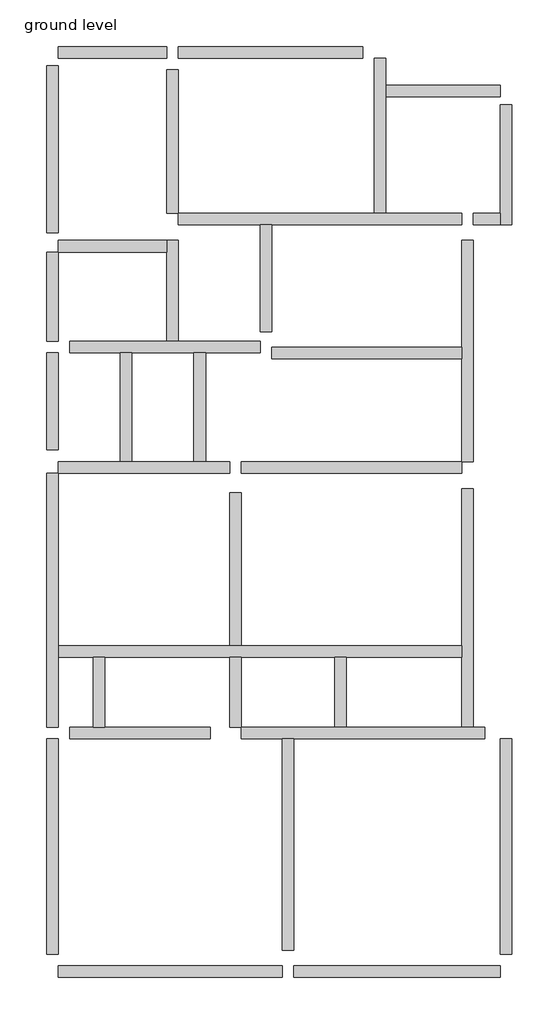
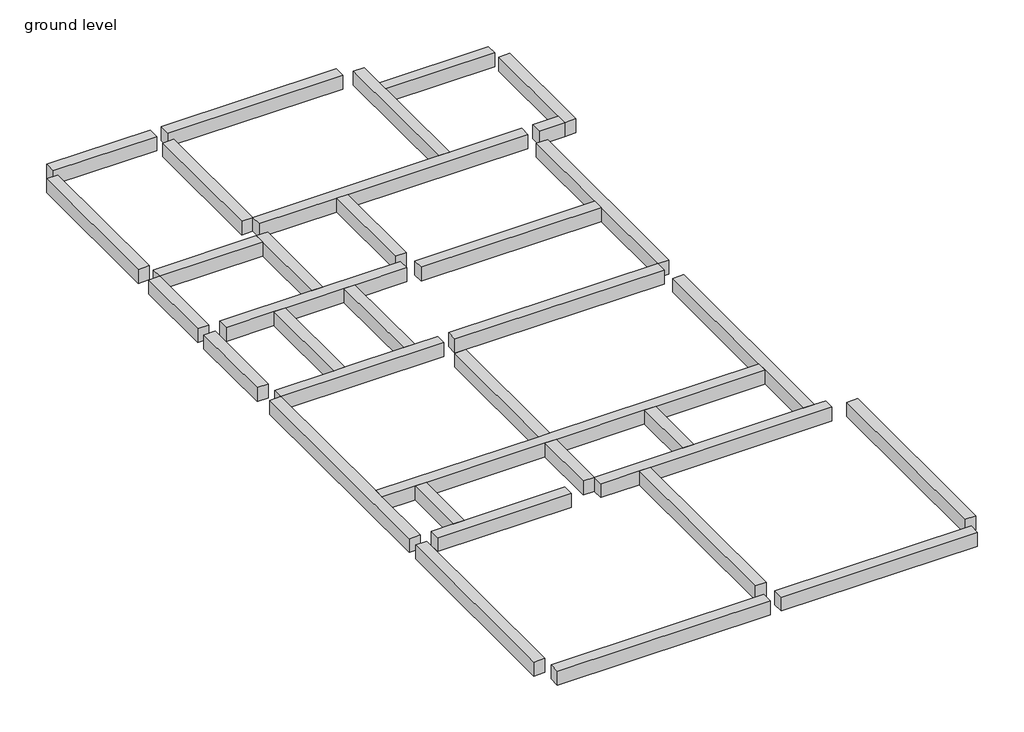
# One storey: 35 beams.
"""IFC4 building model written with IfcOpenShell, lengths in millimetres."""

from ifc_helpers import new_model, si_unit, frame, origin, place, context, project, spatial, polyline, outline, extrude, faceted_brep, element, save

model = new_model("IFC4")

# Units and contexts
model_context = context("Model", 3, world=origin())
ifc_project = project(units=[si_unit("LENGTHUNIT", "METRE", prefix="MILLI")], contexts=[model_context])

# Site, building, storey
site = spatial("IfcSite", under=ifc_project)
building = spatial("IfcBuilding", under=site)
storey = spatial("IfcBuildingStorey", under=building, Name="ground level", Elevation=0.0)

# Beams
placement = place(None, origin())
element("IfcBeam", 1, ObjectType="M_Concrete-Rectangular Beam : 9\" x 12\"", at=placement, inside=storey, context=model_context, shape_type="SweptSolid", body=[
    extrude(outline(polyline([(17883.586814, 18917.5317951), (17654.986814, 18917.5317951), (17654.986814, 22194.1317951), (17883.586814, 22194.1317951), (17883.586814, 18917.5317951)])), frame((0.0, 0.0, -304.8), z_axis=(0.0, 0.0, 1.0), x_axis=(1.0, 0.0, 0.0)), (0.0, 0.0, 1.0), 304.8),
])
element("IfcBeam", 2, ObjectType="M_Concrete-Rectangular Beam : 9\" x 12\"", at=placement, inside=storey, context=model_context, shape_type="SweptSolid", body=[
    extrude(outline(polyline([(20017.186814, 22575.1317951), (20017.186814, 22346.5317951), (17883.586814, 22346.5317951), (17883.586814, 22575.1317951), (20017.186814, 22575.1317951)])), frame((0.0, 0.0, -304.8), z_axis=(0.0, 0.0, 1.0), x_axis=(1.0, 0.0, 0.0)), (0.0, 0.0, 1.0), 304.8),
])
element("IfcBeam", 3, ObjectType="M_Concrete-Rectangular Beam : 9\" x 12\"", at=placement, inside=storey, context=model_context, shape_type="SweptSolid", body=[
    extrude(outline(polyline([(23864.8020345, 22575.1317951), (23864.8020345, 22346.5317951), (20245.786814, 22346.5317951), (20245.786814, 22575.1317951), (23864.8020345, 22575.1317951)])), frame((0.0, 0.0, -304.8), z_axis=(0.0, 0.0, 1.0), x_axis=(1.0, 0.0, 0.0)), (0.0, 0.0, 1.0), 304.8),
])
element("IfcBeam", 4, ObjectType="M_Concrete-Rectangular Beam : 9\" x 12\"", at=placement, inside=storey, context=model_context, shape_type="Brep", body=[
    faceted_brep([(26798.986814, 21432.1317951, 0.0), (26798.986814, 21432.1317951, -304.8), (26570.386814, 21432.1317951, -304.8), (26570.386814, 21432.1317951, 0.0), (26570.386814, 19298.5317951, 0.0), (26570.386814, 19069.9317951, 0.0), (26798.986814, 19069.9317951, 0.0), (26570.386814, 19298.5317951, -304.8), (26570.386814, 19069.9317951, -304.8), (26798.986814, 19069.9317951, -304.8)], [[[0, 1, 2, 3]], [[0, 3, 4, 5, 6]], [[3, 2, 7, 8, 5, 4]], [[2, 1, 9, 8, 7]], [[1, 0, 6, 9]], [[6, 5, 8, 9]]]),
])
element("IfcBeam", 5, ObjectType="M_Concrete-Rectangular Beam : 9\" x 12\"", at=placement, inside=storey, context=model_context, shape_type="SweptSolid", body=[
    extrude(outline(polyline([(26036.986814, 19069.9317951), (26036.986814, 19298.5317951), (26570.386814, 19298.5317951), (26570.386814, 19069.9317951), (26036.986814, 19069.9317951)])), frame((0.0, 0.0, -304.8), z_axis=(0.0, 0.0, 1.0), x_axis=(1.0, 0.0, 0.0)), (0.0, 0.0, 1.0), 304.8),
])
element("IfcBeam", 6, ObjectType="M_Concrete-Rectangular Beam : 9\" x 12\"", at=placement, inside=storey, context=model_context, shape_type="Brep", body=[
    faceted_brep([(20245.786814, 19298.5317951, 0.0), (20245.786814, 19069.9317951, 0.0), (21851.7441916, 19069.9317951, 0.0), (22080.3441916, 19069.9317951, 0.0), (25808.386814, 19069.9317951, 0.0), (25808.386814, 19298.5317951, 0.0), (24318.986814, 19298.5317951, 0.0), (24090.386814, 19298.5317951, 0.0), (20245.786814, 19298.5317951, -304.8), (25808.386814, 19298.5317951, -304.8), (24318.986814, 19298.5317951, -304.8), (24090.386814, 19298.5317951, -304.8), (20245.786814, 19069.9317951, -304.8), (25808.386814, 19069.9317951, -304.8), (22080.3441916, 19069.9317951, -304.8), (21851.7441916, 19069.9317951, -304.8)], [[[0, 1, 2, 3, 4, 5, 6, 7]], [[8, 0, 7, 6, 5, 9, 10, 11]], [[12, 8, 11, 10, 9, 13, 14, 15]], [[1, 12, 15, 14, 13, 4, 3, 2]], [[1, 0, 8, 12]], [[4, 13, 9, 5]]]),
])
element("IfcBeam", 7, ObjectType="M_Concrete-Rectangular Beam : 9\" x 12\"", at=placement, inside=storey, context=model_context, shape_type="SweptSolid", body=[
    extrude(outline(polyline([(20245.786814, 19298.5317951), (20017.186814, 19298.5317951), (20017.186814, 22117.9317951), (20245.786814, 22117.9317951), (20245.786814, 19298.5317951)])), frame((0.0, 0.0, -304.8), z_axis=(0.0, 0.0, 1.0), x_axis=(1.0, 0.0, 0.0)), (0.0, 0.0, 1.0), 304.8),
])
element("IfcBeam", 8, ObjectType="M_Concrete-Rectangular Beam : 9\" x 12\"", at=placement, inside=storey, context=model_context, shape_type="SweptSolid", body=[
    extrude(outline(polyline([(17883.586814, 16783.9317951), (17654.986814, 16783.9317951), (17654.986814, 18536.5317951), (17883.586814, 18536.5317951), (17883.586814, 16783.9317951)])), frame((0.0, 0.0, -304.8), z_axis=(0.0, 0.0, 1.0), x_axis=(1.0, 0.0, 0.0)), (0.0, 0.0, 1.0), 304.8),
])
element("IfcBeam", 9, ObjectType="M_Concrete-Rectangular Beam : 9\" x 12\"", at=placement, inside=storey, context=model_context, shape_type="SweptSolid", body=[
    extrude(outline(polyline([(17883.586814, 14650.3317951), (17654.986814, 14650.3317951), (17654.986814, 16555.3317951), (17883.586814, 16555.3317951), (17883.586814, 14650.3317951)])), frame((0.0, 0.0, -304.8), z_axis=(0.0, 0.0, 1.0), x_axis=(1.0, 0.0, 0.0)), (0.0, 0.0, 1.0), 304.8),
])
element("IfcBeam", 10, ObjectType="M_Concrete-Rectangular Beam : 9\" x 12\"", at=placement, inside=storey, context=model_context, shape_type="Brep", body=[
    faceted_brep([(17654.986814, 9202.0317951, 0.0), (17883.586814, 9202.0317951, 0.0), (17883.586814, 10573.4317951, 0.0), (17883.586814, 10802.0317951, 0.0), (17883.586814, 14193.1317951, 0.0), (17654.986814, 14193.1317951, 0.0), (17654.986814, 9202.0317951, -304.8), (17654.986814, 14193.1317951, -304.8), (17883.586814, 9202.0317951, -304.8), (17883.586814, 14193.1317951, -304.8), (17883.586814, 10802.0317951, -304.8), (17883.586814, 10573.4317951, -304.8)], [[[0, 1, 2, 3, 4, 5]], [[6, 0, 5, 7]], [[8, 6, 7, 9, 10, 11]], [[1, 8, 11, 10, 9, 4, 3, 2]], [[1, 0, 6, 8]], [[4, 9, 7, 5]]]),
])
element("IfcBeam", 11, ObjectType="M_Concrete-Rectangular Beam : 9\" x 12\"", at=placement, inside=storey, context=model_context, shape_type="SweptSolid", body=[
    extrude(outline(polyline([(17883.586814, 4744.3317951), (17654.986814, 4744.3317951), (17654.986814, 8973.4317951), (17883.586814, 8973.4317951), (17883.586814, 4744.3317951)])), frame((0.0, 0.0, -304.8), z_axis=(0.0, 0.0, 1.0), x_axis=(1.0, 0.0, 0.0)), (0.0, 0.0, 1.0), 304.8),
])
element("IfcBeam", 12, ObjectType="M_Concrete-Rectangular Beam : 9\" x 12\"", at=placement, inside=storey, context=model_context, shape_type="SweptSolid", body=[
    extrude(outline(polyline([(22284.136814, 4515.7317951), (22284.136814, 4287.1317951), (17883.586814, 4287.1317951), (17883.586814, 4515.7317951), (22284.136814, 4515.7317951)])), frame((0.0, 0.0, -304.8), z_axis=(0.0, 0.0, 1.0), x_axis=(1.0, 0.0, 0.0)), (0.0, 0.0, 1.0), 304.8),
])
element("IfcBeam", 13, ObjectType="M_Concrete-Rectangular Beam : 9\" x 12\"", at=placement, inside=storey, context=model_context, shape_type="SweptSolid", body=[
    extrude(outline(polyline([(26570.386814, 4515.7317951), (26570.386814, 4287.1317951), (22512.736814, 4287.1317951), (22512.736814, 4515.7317951), (26570.386814, 4515.7317951)])), frame((0.0, 0.0, -304.8), z_axis=(0.0, 0.0, 1.0), x_axis=(1.0, 0.0, 0.0)), (0.0, 0.0, 1.0), 304.8),
])
element("IfcBeam", 14, ObjectType="M_Concrete-Rectangular Beam : 9\" x 12\"", at=placement, inside=storey, context=model_context, shape_type="SweptSolid", body=[
    extrude(outline(polyline([(26570.386814, 8973.4317951), (26798.986814, 8973.4317951), (26798.986814, 4744.3317951), (26570.386814, 4744.3317951), (26570.386814, 8973.4317951)])), frame((0.0, 0.0, -304.8), z_axis=(0.0, 0.0, 1.0), x_axis=(1.0, 0.0, 0.0)), (0.0, 0.0, 1.0), 304.8),
])
element("IfcBeam", 15, ObjectType="M_Concrete-Rectangular Beam : 9\" x 12\"", at=placement, inside=storey, context=model_context, shape_type="Brep", body=[
    faceted_brep([(21483.4441916, 9202.0317951, 0.0), (21483.4441916, 8973.4317951, 0.0), (22284.136814, 8973.4317951, 0.0), (22512.736814, 8973.4317951, 0.0), (26265.586814, 8973.4317951, 0.0), (26265.586814, 9202.0317951, 0.0), (26036.986814, 9202.0317951, 0.0), (25808.386814, 9202.0317951, 0.0), (23541.436814, 9202.0317951, 0.0), (23312.836814, 9202.0317951, 0.0), (21483.4441916, 9202.0317951, -304.8), (26265.586814, 9202.0317951, -304.8), (26036.986814, 9202.0317951, -304.8), (25808.386814, 9202.0317951, -304.8), (23541.436814, 9202.0317951, -304.8), (23312.836814, 9202.0317951, -304.8), (21483.4441916, 8973.4317951, -304.8), (26265.586814, 8973.4317951, -304.8), (22512.736814, 8973.4317951, -304.8), (22284.136814, 8973.4317951, -304.8)], [[[0, 1, 2, 3, 4, 5, 6, 7, 8, 9]], [[10, 0, 9, 8, 7, 6, 5, 11, 12, 13, 14, 15]], [[16, 10, 15, 14, 13, 12, 11, 17, 18, 19]], [[1, 16, 19, 18, 17, 4, 3, 2]], [[4, 17, 11, 5]], [[1, 0, 10, 16]]]),
])
element("IfcBeam", 16, ObjectType="M_Concrete-Rectangular Beam : 9\" x 12\"", at=placement, inside=storey, context=model_context, shape_type="Brep", body=[
    faceted_brep([(18112.186814, 8973.4317951, 0.0), (18112.186814, 9202.0317951, 0.0), (18112.186814, 9202.0317951, -304.8), (18112.186814, 8973.4317951, -304.8), (20873.8441916, 8973.4317951, 0.0), (20873.8441916, 9202.0317951, 0.0), (18796.8015693, 9202.0317951, 0.0), (18568.2015693, 9202.0317951, 0.0), (20873.8441916, 9202.0317951, -304.8), (18796.8015693, 9202.0317951, -304.8), (18568.2015693, 9202.0317951, -304.8), (20873.8441916, 8973.4317951, -304.8)], [[[0, 1, 2, 3]], [[1, 0, 4, 5, 6, 7]], [[2, 1, 7, 6, 5, 8, 9, 10]], [[3, 2, 10, 9, 8, 11]], [[0, 3, 11, 4]], [[4, 11, 8, 5]]]),
])
element("IfcBeam", 17, ObjectType="M_Concrete-Rectangular Beam : 9\" x 12\"", at=placement, inside=storey, context=model_context, shape_type="SweptSolid", body=[
    extrude(outline(polyline([(17883.586814, 18536.5317951), (17883.586814, 18765.1317951), (20017.186814, 18765.1317951), (20017.186814, 18536.5317951), (17883.586814, 18536.5317951)])), frame((0.0, 0.0, -304.8), z_axis=(0.0, 0.0, 1.0), x_axis=(1.0, 0.0, 0.0)), (0.0, 0.0, 1.0), 304.8),
])
element("IfcBeam", 18, ObjectType="M_Concrete-Rectangular Beam : 9\" x 12\"", at=placement, inside=storey, context=model_context, shape_type="Brep", body=[
    faceted_brep([(21851.7441916, 16555.3317951, 0.0), (21851.7441916, 16783.9317951, 0.0), (20245.786814, 16783.9317951, 0.0), (20017.186814, 16783.9317951, 0.0), (18112.186814, 16783.9317951, 0.0), (18112.186814, 16555.3317951, 0.0), (19102.786814, 16555.3317951, 0.0), (19331.386814, 16555.3317951, 0.0), (20550.586814, 16555.3317951, 0.0), (20779.186814, 16555.3317951, 0.0), (21851.7441916, 16555.3317951, -304.8), (18112.186814, 16555.3317951, -304.8), (19102.786814, 16555.3317951, -304.8), (19331.386814, 16555.3317951, -304.8), (20550.586814, 16555.3317951, -304.8), (20779.186814, 16555.3317951, -304.8), (21851.7441916, 16783.9317951, -304.8), (18112.186814, 16783.9317951, -304.8), (20017.186814, 16783.9317951, -304.8), (20245.786814, 16783.9317951, -304.8)], [[[0, 1, 2, 3, 4, 5, 6, 7, 8, 9]], [[10, 0, 9, 8, 7, 6, 5, 11, 12, 13, 14, 15]], [[16, 10, 15, 14, 13, 12, 11, 17, 18, 19]], [[1, 16, 19, 18, 17, 4, 3, 2]], [[4, 17, 11, 5]], [[1, 0, 10, 16]]]),
])
element("IfcBeam", 19, ObjectType="M_Concrete-Rectangular Beam : 9\" x 12\"", at=placement, inside=storey, context=model_context, shape_type="SweptSolid", body=[
    extrude(outline(polyline([(22080.3441916, 16441.0317951), (22080.3441916, 16669.6317951), (25808.386814, 16669.6317951), (25808.386814, 16441.0317951), (22080.3441916, 16441.0317951)])), frame((0.0, 0.0, -304.8), z_axis=(0.0, 0.0, 1.0), x_axis=(1.0, 0.0, 0.0)), (0.0, 0.0, 1.0), 304.8),
])
element("IfcBeam", 20, ObjectType="M_Concrete-Rectangular Beam : 9\" x 12\"", at=placement, inside=storey, context=model_context, shape_type="Brep", body=[
    faceted_brep([(25808.386814, 14421.7317951, 0.0), (26036.986814, 14421.7317951, 0.0), (26036.986814, 18765.1317951, 0.0), (25808.386814, 18765.1317951, 0.0), (25808.386814, 16669.6317951, 0.0), (25808.386814, 16441.0317951, 0.0), (25808.386814, 14421.7317951, -304.8), (25808.386814, 18765.1317951, -304.8), (25808.386814, 16669.6317951, -304.8), (25808.386814, 16441.0317951, -304.8), (26036.986814, 14421.7317951, -304.8), (26036.986814, 18765.1317951, -304.8)], [[[0, 1, 2, 3, 4, 5]], [[6, 0, 5, 4, 3, 7, 8, 9]], [[10, 6, 9, 8, 7, 11]], [[1, 10, 11, 2]], [[2, 11, 7, 3]], [[1, 0, 6, 10]]]),
])
element("IfcBeam", 21, ObjectType="M_Concrete-Rectangular Beam : 9\" x 12\"", at=placement, inside=storey, context=model_context, shape_type="Brep", body=[
    faceted_brep([(26036.986814, 13888.3317951, 0.0), (25808.386814, 13888.3317951, 0.0), (25808.386814, 10802.0317951, 0.0), (25808.386814, 10573.4317951, 0.0), (25808.386814, 9202.0317951, 0.0), (26036.986814, 9202.0317951, 0.0), (25808.386814, 13888.3317951, -304.8), (25808.386814, 10802.0317951, -304.8), (25808.386814, 10573.4317951, -304.8), (25808.386814, 9202.0317951, -304.8), (26036.986814, 13888.3317951, -304.8), (26036.986814, 9202.0317951, -304.8)], [[[0, 1, 2, 3, 4, 5]], [[1, 6, 7, 8, 9, 4, 3, 2]], [[6, 10, 11, 9, 8, 7]], [[10, 0, 5, 11]], [[0, 10, 6, 1]], [[5, 4, 9, 11]]]),
])
element("IfcBeam", 22, ObjectType="M_Concrete-Rectangular Beam : 9\" x 12\"", at=placement, inside=storey, context=model_context, shape_type="Brep", body=[
    faceted_brep([(17883.586814, 10802.0317951, 0.0), (17883.586814, 10573.4317951, 0.0), (18568.2015693, 10573.4317951, 0.0), (18796.8015693, 10573.4317951, 0.0), (21254.8441916, 10573.4317951, 0.0), (21483.4441916, 10573.4317951, 0.0), (23312.836814, 10573.4317951, 0.0), (23541.436814, 10573.4317951, 0.0), (25808.386814, 10573.4317951, 0.0), (25808.386814, 10802.0317951, 0.0), (21483.4441916, 10802.0317951, 0.0), (21254.8441916, 10802.0317951, 0.0), (17883.586814, 10802.0317951, -304.8), (25808.386814, 10802.0317951, -304.8), (21483.4441916, 10802.0317951, -304.8), (21254.8441916, 10802.0317951, -304.8), (17883.586814, 10573.4317951, -304.8), (25808.386814, 10573.4317951, -304.8), (23541.436814, 10573.4317951, -304.8), (23312.836814, 10573.4317951, -304.8), (21483.4441916, 10573.4317951, -304.8), (21254.8441916, 10573.4317951, -304.8), (18796.8015693, 10573.4317951, -304.8), (18568.2015693, 10573.4317951, -304.8)], [[[0, 1, 2, 3, 4, 5, 6, 7, 8, 9, 10, 11]], [[12, 0, 11, 10, 9, 13, 14, 15]], [[16, 12, 15, 14, 13, 17, 18, 19, 20, 21, 22, 23]], [[1, 16, 23, 22, 21, 20, 19, 18, 17, 8, 7, 6, 5, 4, 3, 2]], [[1, 0, 12, 16]], [[9, 8, 17, 13]]]),
])
element("IfcBeam", 23, ObjectType="M_Concrete-Rectangular Beam : 9\" x 12\"", at=placement, inside=storey, context=model_context, shape_type="SweptSolid", body=[
    extrude(outline(polyline([(18796.8015693, 9202.0317951), (18568.2015693, 9202.0317951), (18568.2015693, 10573.4317951), (18796.8015693, 10573.4317951), (18796.8015693, 9202.0317951)])), frame((0.0, 0.0, -304.8), z_axis=(0.0, 0.0, 1.0), x_axis=(1.0, 0.0, 0.0)), (0.0, 0.0, 1.0), 304.8),
])
element("IfcBeam", 24, ObjectType="M_Concrete-Rectangular Beam : 9\" x 12\"", at=placement, inside=storey, context=model_context, shape_type="SweptSolid", body=[
    extrude(outline(polyline([(21254.8441916, 10573.4317951), (21483.4441916, 10573.4317951), (21483.4441916, 9202.0317951), (21254.8441916, 9202.0317951), (21254.8441916, 10573.4317951)])), frame((0.0, 0.0, -304.8), z_axis=(0.0, 0.0, 1.0), x_axis=(1.0, 0.0, 0.0)), (0.0, 0.0, 1.0), 304.8),
])
element("IfcBeam", 25, ObjectType="M_Concrete-Rectangular Beam : 9\" x 12\"", at=placement, inside=storey, context=model_context, shape_type="SweptSolid", body=[
    extrude(outline(polyline([(21254.8441916, 13812.1317951), (21483.4441916, 13812.1317951), (21483.4441916, 10802.0317951), (21254.8441916, 10802.0317951), (21254.8441916, 13812.1317951)])), frame((0.0, 0.0, -304.8), z_axis=(0.0, 0.0, 1.0), x_axis=(1.0, 0.0, 0.0)), (0.0, 0.0, 1.0), 304.8),
])
element("IfcBeam", 26, ObjectType="M_Concrete-Rectangular Beam : 9\" x 12\"", at=placement, inside=storey, context=model_context, shape_type="Brep", body=[
    faceted_brep([(21254.8441916, 14193.1317951, 0.0), (21254.8441916, 14193.1317951, -304.8), (21254.8441916, 14421.7317951, -304.8), (21254.8441916, 14421.7317951, 0.0), (20779.186814, 14421.7317951, 0.0), (20550.586814, 14421.7317951, 0.0), (19331.386814, 14421.7317951, 0.0), (19102.786814, 14421.7317951, 0.0), (17883.586814, 14421.7317951, 0.0), (17883.586814, 14193.1317951, 0.0), (20779.186814, 14421.7317951, -304.8), (20550.586814, 14421.7317951, -304.8), (19331.386814, 14421.7317951, -304.8), (19102.786814, 14421.7317951, -304.8), (17883.586814, 14421.7317951, -304.8), (17883.586814, 14193.1317951, -304.8)], [[[0, 1, 2, 3]], [[0, 3, 4, 5, 6, 7, 8, 9]], [[3, 2, 10, 11, 12, 13, 14, 8, 7, 6, 5, 4]], [[2, 1, 15, 14, 13, 12, 11, 10]], [[1, 0, 9, 15]], [[9, 8, 14, 15]]]),
])
element("IfcBeam", 27, ObjectType="M_Concrete-Rectangular Beam : 9\" x 12\"", at=placement, inside=storey, context=model_context, shape_type="SweptSolid", body=[
    extrude(outline(polyline([(19102.786814, 16555.3317951), (19331.386814, 16555.3317951), (19331.386814, 14421.7317951), (19102.786814, 14421.7317951), (19102.786814, 16555.3317951)])), frame((0.0, 0.0, -304.8), z_axis=(0.0, 0.0, 1.0), x_axis=(1.0, 0.0, 0.0)), (0.0, 0.0, 1.0), 304.8),
])
element("IfcBeam", 28, ObjectType="M_Concrete-Rectangular Beam : 9\" x 12\"", at=placement, inside=storey, context=model_context, shape_type="SweptSolid", body=[
    extrude(outline(polyline([(20779.186814, 14421.7317951), (20550.586814, 14421.7317951), (20550.586814, 16555.3317951), (20779.186814, 16555.3317951), (20779.186814, 14421.7317951)])), frame((0.0, 0.0, -304.8), z_axis=(0.0, 0.0, 1.0), x_axis=(1.0, 0.0, 0.0)), (0.0, 0.0, 1.0), 304.8),
])
element("IfcBeam", 29, ObjectType="M_Concrete-Rectangular Beam : 9\" x 12\"", at=placement, inside=storey, context=model_context, shape_type="Brep", body=[
    faceted_brep([(20245.786814, 18765.1317951, 0.0), (20017.186814, 18765.1317951, 0.0), (20017.186814, 18536.5317951, 0.0), (20017.186814, 16783.9317951, 0.0), (20245.786814, 16783.9317951, 0.0), (20017.186814, 18765.1317951, -304.8), (20017.186814, 18536.5317951, -304.8), (20017.186814, 16783.9317951, -304.8), (20245.786814, 18765.1317951, -304.8), (20245.786814, 16783.9317951, -304.8)], [[[0, 1, 2, 3, 4]], [[1, 5, 6, 7, 3, 2]], [[5, 8, 9, 7, 6]], [[8, 0, 4, 9]], [[0, 8, 5, 1]], [[4, 3, 7, 9]]]),
])
element("IfcBeam", 30, ObjectType="M_Concrete-Rectangular Beam : 9\" x 12\"", at=placement, inside=storey, context=model_context, shape_type="SweptSolid", body=[
    extrude(outline(polyline([(22080.3441916, 16974.4317951), (21851.7441916, 16974.4317951), (21851.7441916, 19069.9317951), (22080.3441916, 19069.9317951), (22080.3441916, 16974.4317951)])), frame((0.0, 0.0, -304.8), z_axis=(0.0, 0.0, 1.0), x_axis=(1.0, 0.0, 0.0)), (0.0, 0.0, 1.0), 304.8),
])
element("IfcBeam", 31, ObjectType="M_Concrete-Rectangular Beam : 9\" x 12\"", at=placement, inside=storey, context=model_context, shape_type="SweptSolid", body=[
    extrude(outline(polyline([(24322.486814, 21584.5317951), (24322.486814, 21813.1317951), (26570.386814, 21813.1317951), (26570.386814, 21584.5317951), (24322.486814, 21584.5317951)])), frame((0.0, 0.0, -304.8), z_axis=(0.0, 0.0, 1.0), x_axis=(1.0, 0.0, 0.0)), (0.0, 0.0, 1.0), 304.8),
])
element("IfcBeam", 32, ObjectType="M_Concrete-Rectangular Beam : 9\" x 12\"", at=placement, inside=storey, context=model_context, shape_type="SweptSolid", body=[
    extrude(outline(polyline([(24090.386814, 22346.5317951), (24318.986814, 22346.5317951), (24318.986814, 19298.5317951), (24090.386814, 19298.5317951), (24090.386814, 22346.5317951)])), frame((0.0, 0.0, -304.8), z_axis=(0.0, 0.0, 1.0), x_axis=(1.0, 0.0, 0.0)), (0.0, 0.0, 1.0), 304.8),
])
element("IfcBeam", 33, ObjectType="M_Concrete-Rectangular Beam : 9\" x 12\"", at=placement, inside=storey, context=model_context, shape_type="SweptSolid", body=[
    extrude(outline(polyline([(23541.436814, 9202.0317951), (23312.836814, 9202.0317951), (23312.836814, 10573.4317951), (23541.436814, 10573.4317951), (23541.436814, 9202.0317951)])), frame((0.0, 0.0, -304.8), z_axis=(0.0, 0.0, 1.0), x_axis=(1.0, 0.0, 0.0)), (0.0, 0.0, 1.0), 304.8),
])
element("IfcBeam", 34, ObjectType="M_Concrete-Rectangular Beam : 9\" x 12\"", at=placement, inside=storey, context=model_context, shape_type="SweptSolid", body=[
    extrude(outline(polyline([(22512.736814, 4820.5317951), (22284.136814, 4820.5317951), (22284.136814, 8973.4317951), (22512.736814, 8973.4317951), (22512.736814, 4820.5317951)])), frame((0.0, 0.0, -304.8), z_axis=(0.0, 0.0, 1.0), x_axis=(1.0, 0.0, 0.0)), (0.0, 0.0, 1.0), 304.8),
])
element("IfcBeam", 35, ObjectType="M_Concrete-Rectangular Beam : 9\" x 12\"", at=placement, inside=storey, context=model_context, shape_type="SweptSolid", body=[
    extrude(outline(polyline([(25808.386814, 14421.7317951), (25808.386814, 14193.1317951), (21483.4441916, 14193.1317951), (21483.4441916, 14421.7317951), (25808.386814, 14421.7317951)])), frame((0.0, 0.0, -304.8), z_axis=(0.0, 0.0, 1.0), x_axis=(1.0, 0.0, 0.0)), (0.0, 0.0, 1.0), 304.8),
])

save(model, "model.ifc")

# Revit data of these elements
# Type "M_Concrete-Rectangular Beam : 9\" x 12\""
#   Length [instance default] = 1524 mm
#   b = 228.6 mm
#   h = 304.8 mm
#   Structural Material [instance default] = Concrete, Cast-in-Place gray
#   Assembly Code = ""
# Elements 1, 2, 3, 4, 5, 6, 7, 8, 9, 10, 11, 12, 13, 14, 15, 16, 17, 18, 19, 20, 21, 22, 23, 24, 25, 26, 27, 28, 29, 30, 31, 32, 33, 34, 35 (IfcBeam, "M_Concrete-Rectangular Beam : 9\" x 12\"")
#   Structural Material = Concrete, Cast-in-Place gray
#   Phase Created = New Construction
#   Materials on its faces: "Concrete, Cast-in-Place gray"
# Materials
#   "Concrete, Cast-in-Place gray": class "Concrete", colour RGB 192 192 192, transparency 0, Description = "Cast-in-place concrete", Cost = 0
